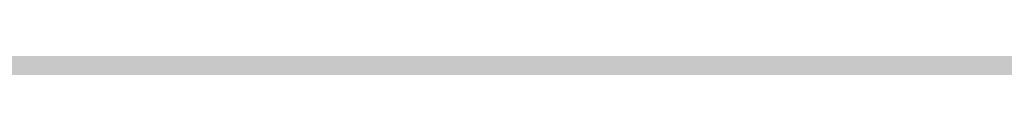
# Model space of a CAD drawing. Units: millimetres. Extents: x 0 to 2267, y 0 to 1823.
# Tile 152 of 256: x 1833.606 to 1838.83, y 1127.355 to 1127.393. Entities that reach past the tile are written whole.
import ezdxf

# ---------------------------------------------------------------- set-up
doc = ezdxf.new("R2010")
doc.units = ezdxf.units.MM
doc.header["$MEASUREMENT"] = 0
doc.layers.add('M-DIMS', color=2, linetype='Continuous', lineweight=25)
doc.layers.add('M-HATC', color=252, linetype='Continuous', lineweight=18)
doc.styles.get("Standard").update_dxf_attribs({"font": 'arial.ttf'})
doc.dimstyles.get("Standard").update_dxf_attribs({"dimtxt": 7, "dimasz": 4, "dimexe": 0.18, "dimexo": 0.0625, "dimgap": 0.09, "dimtad": 0, "dimdec": 0, "dimzin": 0, "dimdsep": 46, "dimtxsty": 'Standard', "dimcen": 0.09, "dimadec": 0, "dimazin": 0, "dimtfac": 1, "dimtdec": 0, "dimtofl": 0, "dimtmove": 0, "dimatfit": 3, "dimfxl": 1, "dimtolj": 1, "dimtzin": 0, "dimarcsym": 0})

# ---------------------------------------------------------------- blocks, each defined once
blk = doc.blocks.new('*D1')
at = {"layer": 'Defpoints', "color": 0, "transparency": 16777216}
for p in [(1593.4289, 1127.4171), (1843.4289, 1127.4171), (1843.4289, 955.6278)]:
    blk.add_point(p, dxfattribs=at)
at = {"layer": 'M-DIMS', "color": 0, "lineweight": -2, "transparency": 16777216}
for p, q in [((1593.4289, 1127.3546), (1593.4289, 955.4478)), ((1843.4289, 1127.3546), (1843.4289, 955.4478)), ((1597.4289, 955.6278), (1710.5582, 955.6278)), ((1839.4289, 955.6278), (1726.2996, 955.6278))]:
    blk.add_line(p, q, dxfattribs=at)
at = {"layer": 'M-DIMS', "color": 0, "transparency": 16777216}
for points in [[(1597.4289, 956.2944), (1597.4289, 954.9611), (1593.4289, 955.6278)], [(1839.4289, 956.2944), (1839.4289, 954.9611), (1843.4289, 955.6278)]]:
    blk.add_solid(points, dxfattribs=at)
at = {"layer": 'M-DIMS', "color": 0, "transparency": 16777216, "insert": (1718.4289, 955.6278), "char_height": 7, "attachment_point": 5}
blk.add_mtext('\\A1;250', dxfattribs=at)

msp = doc.modelspace()

# ---------------------------------------------------------------- hatches: boundary and pattern name
at = {"layer": 'M-HATC'}
h = msp.add_hatch(color=256, dxfattribs=at)
h.dxf.hatch_style = 1
h.paths.add_polyline_path([(2055.771, 1603.062), (1381.0868, 1603.062), (1381.0868, 1598.062), (2055.771, 1598.062)])
h.paths.add_polyline_path([(2055.771, 1598.062), (1381.0868, 1598.062), (1381.0868, 1593.062), (2055.771, 1593.062)])
h.paths.add_polyline_path([(2051.3074, 1536.7609), (1385.5504, 1536.7609), (1385.5504, 1526.7609), (1387.5504, 1526.7609), (1388.5366, 1525.0528), (1385.3319, 1521.2335), (1385.3319, 1521.2226), (2050.2542, 1522.7491), (2048.3212, 1525.0528), (2049.3074, 1526.7609), (2051.3074, 1526.7609)])
edge = h.paths.add_edge_path()
edge.add_arc((1847.5345, 1379.1492), 135, 222.603061, 222.890851, ccw=False)
edge.add_line((1748.1663, 1287.7656), (1683.0921, 1287.7656))
edge.add_arc((1583.7239, 1379.1492), 135, 317.109149, 317.396939, ccw=False)
edge.add_arc((1678.9686, 1290.6707), 5, 222.8909, 317.1091, ccw=False)
edge.add_arc((1774.2133, 1379.1492), 135, 222.603061, 222.890851, ccw=False)
edge.add_line((1674.8451, 1287.7656), (1609.7709, 1287.7656))
edge.add_arc((1510.4027, 1379.1492), 135, 317.109149, 317.396939, ccw=False)
edge.add_arc((1605.6474, 1290.6707), 5, 222.8909, 317.1091, ccw=False)
edge.add_arc((1700.8921, 1379.1492), 135, 222.603061, 222.890851, ccw=False)
edge.add_line((1601.5239, 1287.7656), (1536.4497, 1287.7656))
edge.add_arc((1437.0815, 1379.1492), 135, 317.109149, 317.396939, ccw=False)
edge.add_arc((1532.3262, 1290.6707), 5, 222.8909, 317.1091, ccw=False)
edge.add_arc((1627.5709, 1379.1492), 135, 222.603061, 222.890851, ccw=False)
edge.add_line((1528.2027, 1287.7656), (1505.9289, 1287.7656))
edge.add_spline(control_points=[(1505.9289, 1287.7656), (1504.2622, 1287.7656), (1504.2622, 1282.7656), (1505.9289, 1282.7656)], knot_values=[0, 0, 0, 0, 5, 5, 5, 5], degree=3, periodic=0)
edge.add_line((1505.9289, 1282.7656), (1930.9289, 1282.7656))
edge.add_spline(control_points=[(1930.9289, 1282.7656), (1932.5956, 1282.7656), (1932.5956, 1287.7656), (1930.9289, 1287.7656)], knot_values=[0, 0, 0, 0, 5, 5, 5, 5], degree=3, periodic=0)
edge.add_line((1930.9289, 1287.7656), (1903.0557, 1287.7656))
edge.add_arc((1803.6875, 1379.1492), 135, 317.109149, 317.396939, ccw=False)
edge.add_arc((1898.9322, 1290.6707), 5, 222.8909, 317.1091, ccw=False)
edge.add_arc((1994.1769, 1379.1492), 135, 222.603061, 222.890851, ccw=False)
edge.add_line((1894.8087, 1287.7656), (1829.7345, 1287.7656))
edge.add_arc((1730.3663, 1379.1492), 135, 317.109149, 317.396939, ccw=False)
edge.add_arc((1825.611, 1290.6707), 5, 222.8909, 317.1091, ccw=False)
edge.add_arc((1920.8557, 1379.1492), 135, 222.603061, 222.890851, ccw=False)
edge.add_line((1821.4875, 1287.7656), (1756.4133, 1287.7656))
edge.add_arc((1657.0451, 1379.1492), 135, 317.109149, 317.396939, ccw=False)
edge.add_arc((1752.2898, 1290.6707), 5, 222.8909, 317.1091, ccw=False)
edge = h.paths.add_edge_path()
edge.add_spline(control_points=[(1843.4289, 1227.2475), (1845.0956, 1227.2475), (1845.0956, 1232.2475), (1843.4289, 1232.2475)], knot_values=[0, 0, 0, 0, 5, 5, 5, 5], degree=3, periodic=0)
edge.add_line((1843.4289, 1232.2475), (1593.4289, 1232.2475))
edge.add_spline(control_points=[(1593.4289, 1232.2475), (1591.7622, 1232.2475), (1591.7622, 1227.2475), (1593.4289, 1227.2475)], knot_values=[0, 0, 0, 0, 5, 5, 5, 5], degree=3, periodic=0)
edge.add_line((1593.4289, 1227.2475), (1843.4289, 1227.2475))
h.paths.add_polyline_path([(1905.9289, 1127.4171), (1530.9289, 1127.4171, 0.414214), (1520.9289, 1117.4171), (1530.9289, 1117.4171), (1915.9289, 1117.4171, 0.414214)])
edge = h.paths.add_edge_path()
edge.add_arc((1397.0858, 1498.4078), 12.7299, 90.78215, 190.87871, ccw=False)
edge.add_line((1396.912, 1511.1365), (1428.0097, 1511.3488))
edge.add_line((1428.0097, 1511.3488), (1433.0097, 1511.3488))
edge.add_line((1433.0097, 1511.3488), (1434.439, 1511.3488))
edge.add_arc((1419.474, 1498.0804), 20, 41.561, 74.08211)
edge.add_line((1424.9592, 1517.3135), (1399.9351, 1517.2561))
edge.add_spline(control_points=[(1399.9307, 1517.2561), (1399.884, 1517.2131), (1399.8328, 1517.1689), (1399.7774, 1517.1236)], knot_values=[11.567499, 11.567499, 11.567499, 11.567499, 11.814249, 11.814249, 11.814249, 11.814249], degree=3, periodic=0)
edge.add_spline(control_points=[(1399.6328, 1517.0099), (1399.5831, 1516.9721), (1399.5307, 1516.9338), (1399.4759, 1516.8947)], knot_values=[11.167718, 11.167718, 11.167718, 11.167718, 11.365188, 11.365188, 11.365188, 11.365188], degree=3, periodic=0)
edge.add_spline(control_points=[(1399.3398, 1516.8001), (1399.1514, 1516.6719), (1398.9384, 1516.5377), (1398.704, 1516.3994)], knot_values=[10.376405, 10.376405, 10.376405, 10.376405, 11.00994, 11.00994, 11.00994, 11.00994], degree=3, periodic=0)
edge.add_spline(control_points=[(1398.6572, 1516.3719), (1398.5789, 1516.326), (1398.4983, 1516.2797), (1398.4155, 1516.2331)], knot_values=[10.125175, 10.125175, 10.125175, 10.125175, 10.334406, 10.334406, 10.334406, 10.334406], degree=3, periodic=0)
edge.add_spline(control_points=[(1398.2642, 1516.1487), (1398.196, 1516.1111), (1398.1263, 1516.0732), (1398.0555, 1516.0351)], knot_values=[9.832246, 9.832246, 9.832246, 9.832246, 9.999658, 9.999658, 9.999658, 9.999658], degree=3, periodic=0)
edge.add_spline(control_points=[(1397.9987, 1516.0048), (1397.7312, 1515.8621), (1397.446, 1515.7171), (1397.1466, 1515.5714)], knot_values=[9.161808, 9.161808, 9.161808, 9.161808, 9.787769, 9.787769, 9.787769, 9.787769], degree=3, periodic=0)
edge.add_spline(control_points=[(1397.1466, 1515.5714), (1396.8418, 1515.423), (1396.5222, 1515.274), (1396.1914, 1515.1262)], knot_values=[8.524455, 8.524455, 8.524455, 8.524455, 9.161808, 9.161808, 9.161808, 9.161808], degree=3, periodic=0)
edge.add_spline(control_points=[(1396.0777, 1515.0756), (1395.9854, 1515.0348), (1395.8922, 1514.994), (1395.7983, 1514.9534)], knot_values=[8.275193, 8.275193, 8.275193, 8.275193, 8.451726, 8.451726, 8.451726, 8.451726], degree=3, periodic=0)
edge.add_spline(control_points=[(1395.6018, 1514.8691), (1395.4997, 1514.8257), (1395.3968, 1514.7824), (1395.2932, 1514.7394)], knot_values=[7.962917, 7.962917, 7.962917, 7.962917, 8.152764, 8.152764, 8.152764, 8.152764], degree=3, periodic=0)
edge.add_spline(control_points=[(1395.2116, 1514.7057), (1394.8278, 1514.5475), (1394.4345, 1514.3929), (1394.0364, 1514.2442)], knot_values=[7.21254, 7.21254, 7.21254, 7.21254, 7.913148, 7.913148, 7.913148, 7.913148], degree=3, periodic=0)
edge.add_spline(control_points=[(1394.0364, 1514.2442), (1393.7076, 1514.1214), (1393.3754, 1514.0027), (1393.0427, 1513.8895)], knot_values=[6.633733, 6.633733, 6.633733, 6.633733, 7.21254, 7.21254, 7.21254, 7.21254], degree=3, periodic=0)
edge.add_spline(control_points=[(1392.8214, 1513.815), (1392.7198, 1513.7812), (1392.6181, 1513.7479), (1392.5166, 1513.7152)], knot_values=[6.328796, 6.328796, 6.328796, 6.328796, 6.505493, 6.505493, 6.505493, 6.505493], degree=3, periodic=0)
edge.add_spline(control_points=[(1392.5166, 1513.7152), (1392.3187, 1513.6515), (1392.1212, 1513.59), (1391.9244, 1513.531)], knot_values=[5.984605, 5.984605, 5.984605, 5.984605, 6.328796, 6.328796, 6.328796, 6.328796], degree=3, periodic=0)
edge.add_spline(control_points=[(1391.7915, 1513.4915), (1391.3122, 1513.3501), (1390.8384, 1513.2239), (1390.3784, 1513.1171)], knot_values=[5.066697, 5.066697, 5.066697, 5.066697, 5.907055, 5.907055, 5.907055, 5.907055], degree=3, periodic=0)
edge.add_spline(control_points=[(1390.3784, 1513.1171), (1390.1797, 1513.071), (1389.9836, 1513.0284), (1389.7907, 1512.9899)], knot_values=[4.70367, 4.70367, 4.70367, 4.70367, 5.066695, 5.066695, 5.066695, 5.066695], degree=3, periodic=0)
edge.add_spline(control_points=[(1389.422, 1512.9204), (1389.2459, 1512.8892), (1389.0729, 1512.8617), (1388.9036, 1512.8381)], knot_values=[4.130571, 4.130571, 4.130571, 4.130571, 4.469816, 4.469816, 4.469816, 4.469816], degree=3, periodic=0)
edge.add_spline(control_points=[(1388.9036, 1512.8381), (1388.591, 1512.7946), (1388.2911, 1512.7644), (1388.0071, 1512.7494)], knot_values=[3.504031, 3.504031, 3.504031, 3.504031, 4.130571, 4.130571, 4.130571, 4.130571], degree=3, periodic=0)
edge.add_spline(control_points=[(1387.9356, 1512.7459), (1387.8538, 1512.7423), (1387.7733, 1512.74), (1387.6944, 1512.739)], knot_values=[3.268866, 3.268866, 3.268866, 3.268866, 3.451164, 3.451164, 3.451164, 3.451164], degree=3, periodic=0)
edge.add_spline(control_points=[(1387.3351, 1512.7443), (1387.2076, 1512.7499), (1387.0847, 1512.7597), (1386.967, 1512.7739)], knot_values=[2.670686, 2.670686, 2.670686, 2.670686, 2.984, 2.984, 2.984, 2.984], degree=3, periodic=0)
edge.add_spline(control_points=[(1386.8327, 1512.7922), (1386.8209, 1512.7941), (1386.8092, 1512.7959), (1386.7975, 1512.7979)], knot_values=[2.516981, 2.516981, 2.516981, 2.516981, 2.549528, 2.549528, 2.549528, 2.549528], degree=3, periodic=0)
edge.add_spline(control_points=[(1386.4526, 1512.8735), (1386.4257, 1512.881), (1386.3993, 1512.889), (1386.3733, 1512.8972)], knot_values=[2.095869, 2.095869, 2.095869, 2.095869, 2.17941, 2.17941, 2.17941, 2.17941], degree=3, periodic=0)
edge.add_spline(control_points=[(1386.0691, 1513.0189), (1386.0634, 1513.0217), (1386.0577, 1513.0246), (1386.052, 1513.0275)], knot_values=[1.72453, 1.72453, 1.72453, 1.72453, 1.745933, 1.745933, 1.745933, 1.745933], degree=3, periodic=0)
edge.add_arc((1399.474, 1498.0804), 20, 131.82432, 180)
edge.add_arc((1630.3336, 1505.5484), 250.9708, 181.705176, 236.427975)
edge.add_arc((1605.3399, 1483.3044), 218.7822, 238.660829, 243.34961)
edge.add_arc((1647.0911, 1510.3592), 262.8986, 183.129836, 237.853442, ccw=False)
h.paths.add_polyline_path([(1406.5369, 1391.9644, 0.149382), (1491.5506, 1296.4418, -0.129517)], flags=17)
edge = h.paths.add_edge_path()
edge.add_arc((2037.3838, 1498.0804), 20, 0, 48.26587)
edge.add_spline(control_points=[(2050.6973, 1513.0052), (2050.6512, 1512.9847), (2050.6034, 1512.9655), (2050.5539, 1512.9477)], knot_values=[1.835652, 1.835652, 1.835652, 1.835652, 2.000781, 2.000781, 2.000781, 2.000781], degree=3, periodic=0)
edge.add_spline(control_points=[(2050.4616, 1512.9166), (2050.479, 1512.9221), (2050.4963, 1512.9277), (2050.5133, 1512.9335)], knot_values=[2.045477, 2.045477, 2.045477, 2.045477, 2.101389, 2.101389, 2.101389, 2.101389], degree=3, periodic=0)
edge.add_spline(control_points=[(2050.129, 1512.8342), (2050.1984, 1512.8473), (2050.2657, 1512.8623), (2050.3308, 1512.8792)], knot_values=[2.237629, 2.237629, 2.237629, 2.237629, 2.435841, 2.435841, 2.435841, 2.435841], degree=3, periodic=0)
edge.add_spline(control_points=[(2050.0946, 1512.8278), (2050.1061, 1512.8299), (2050.1176, 1512.832), (2050.129, 1512.8342)], knot_values=[2.435841, 2.435841, 2.435841, 2.435841, 2.468321, 2.468321, 2.468321, 2.468321], degree=3, periodic=0)
edge.add_spline(control_points=[(2049.7843, 1512.7851), (2049.8552, 1512.7922), (2049.9243, 1512.8008), (2049.9917, 1512.8109)], knot_values=[2.563852, 2.563852, 2.563852, 2.563852, 2.748541, 2.748541, 2.748541, 2.748541], degree=3, periodic=0)
edge.add_spline(control_points=[(2049.4052, 1512.7617), (2049.5364, 1512.7653), (2049.6629, 1512.773), (2049.7843, 1512.7851)], knot_values=[2.748541, 2.748541, 2.748541, 2.748541, 3.064882, 3.064882, 3.064882, 3.064882], degree=3, periodic=0)
edge.add_spline(control_points=[(2049.1698, 1512.7597), (2049.2336, 1512.7591), (2049.2965, 1512.7594), (2049.3584, 1512.7606)], knot_values=[3.102309, 3.102309, 3.102309, 3.102309, 3.2503, 3.2503, 3.2503, 3.2503], degree=3, periodic=0)
edge.add_spline(control_points=[(2048.8573, 1512.7691), (2048.9638, 1512.7638), (2049.068, 1512.7606), (2049.1698, 1512.7597)], knot_values=[3.2503, 3.2503, 3.2503, 3.2503, 3.486069, 3.486069, 3.486069, 3.486069], degree=3, periodic=0)
edge.add_spline(control_points=[(2048.6924, 1512.7789), (2048.3729, 1512.8009), (2048.0345, 1512.8411), (2047.6817, 1512.897)], knot_values=[3.606429, 3.606429, 3.606429, 3.606429, 4.2989, 4.2989, 4.2989, 4.2989], degree=3, periodic=0)
edge.add_spline(control_points=[(2047.6817, 1512.897), (2047.5458, 1512.9185), (2047.4077, 1512.9424), (2047.2678, 1512.9685)], knot_values=[4.2989, 4.2989, 4.2989, 4.2989, 4.565769, 4.565769, 4.565769, 4.565769], degree=3, periodic=0)
edge.add_spline(control_points=[(2047.2678, 1512.9685), (2047.1449, 1512.9914), (2047.0207, 1513.016), (2046.8951, 1513.0422)], knot_values=[4.565769, 4.565769, 4.565769, 4.565769, 4.799971, 4.799971, 4.799971, 4.799971], degree=3, periodic=0)
edge.add_spline(control_points=[(2046.8951, 1513.0422), (2046.5286, 1513.1188), (2046.1513, 1513.209), (2045.7676, 1513.3107)], knot_values=[4.799971, 4.799971, 4.799971, 4.799971, 5.483718, 5.483718, 5.483718, 5.483718], degree=3, periodic=0)
edge.add_spline(control_points=[(2045.7676, 1513.3107), (2045.3724, 1513.4154), (2044.9704, 1513.5322), (2044.5662, 1513.6588)], knot_values=[5.483718, 5.483718, 5.483718, 5.483718, 6.187866, 6.187866, 6.187866, 6.187866], degree=3, periodic=0)
edge.add_spline(control_points=[(2044.5662, 1513.6588), (2044.4149, 1513.7061), (2044.2633, 1513.7549), (2044.1116, 1513.8048)], knot_values=[6.187866, 6.187866, 6.187866, 6.187866, 6.451551, 6.451551, 6.451551, 6.451551], degree=3, periodic=0)
edge.add_spline(control_points=[(2044.1116, 1513.8048), (2043.9967, 1513.8427), (2043.8817, 1513.8813), (2043.7668, 1513.9205)], knot_values=[6.451551, 6.451551, 6.451551, 6.451551, 6.651434, 6.651434, 6.651434, 6.651434], degree=3, periodic=0)
edge.add_spline(control_points=[(2043.7668, 1513.9205), (2043.3716, 1514.0554), (2042.9774, 1514.1979), (2042.5886, 1514.3458)], knot_values=[6.651434, 6.651434, 6.651434, 6.651434, 7.338879, 7.338879, 7.338879, 7.338879], degree=3, periodic=0)
edge.add_spline(control_points=[(2042.5886, 1514.3458), (2042.1643, 1514.5071), (2041.7465, 1514.6749), (2041.3409, 1514.846)], knot_values=[7.338879, 7.338879, 7.338879, 7.338879, 8.089209, 8.089209, 8.089209, 8.089209], degree=3, periodic=0)
edge.add_spline(control_points=[(2041.3409, 1514.846), (2041.1028, 1514.9465), (2040.869, 1515.0481), (2040.6405, 1515.1502)], knot_values=[8.089209, 8.089209, 8.089209, 8.089209, 8.529587, 8.529587, 8.529587, 8.529587], degree=3, periodic=0)
edge.add_spline(control_points=[(2040.51, 1515.2089), (2040.0824, 1515.4022), (2039.6747, 1515.5971), (2039.295, 1515.7894)], knot_values=[8.613818, 8.613818, 8.613818, 8.613818, 9.44571, 9.44571, 9.44571, 9.44571], degree=3, periodic=0)
edge.add_spline(control_points=[(2039.295, 1515.7894), (2039.0618, 1515.9075), (2038.8391, 1516.0246), (2038.6288, 1516.1398)], knot_values=[9.44571, 9.44571, 9.44571, 9.44571, 9.956404, 9.956404, 9.956404, 9.956404], degree=3, periodic=0)
edge.add_spline(control_points=[(2038.6288, 1516.1398), (2038.5187, 1516.2001), (2038.4121, 1516.2598), (2038.309, 1516.3189)], knot_values=[9.956404, 9.956404, 9.956404, 9.956404, 10.223542, 10.223542, 10.223542, 10.223542], degree=3, periodic=0)
edge.add_spline(control_points=[(2038.309, 1516.3189), (2038.2138, 1516.3735), (2038.1216, 1516.4276), (2038.0328, 1516.481)], knot_values=[10.223542, 10.223542, 10.223542, 10.223542, 10.47051, 10.47051, 10.47051, 10.47051], degree=3, periodic=0)
edge.add_spline(control_points=[(2038.0328, 1516.481), (2037.7855, 1516.6296), (2037.5639, 1516.773), (2037.3722, 1516.909)], knot_values=[10.47051, 10.47051, 10.47051, 10.47051, 11.15767, 11.15767, 11.15767, 11.15767], degree=3, periodic=0)
edge.add_spline(control_points=[(2037.3722, 1516.909), (2037.2789, 1516.9752), (2037.1927, 1517.0396), (2037.1142, 1517.102)], knot_values=[11.15767, 11.15767, 11.15767, 11.15767, 11.49227, 11.49227, 11.49227, 11.49227], degree=3, periodic=0)
edge.add_spline(control_points=[(2036.8564, 1517.3259), (2036.9148, 1517.2692), (2036.9814, 1517.2103), (2037.0557, 1517.1492)], knot_values=[11.577341, 11.577341, 11.577341, 11.577341, 11.91035, 11.91035, 11.91035, 11.91035], degree=3, periodic=0)
edge.add_spline(control_points=[(2036.8074, 1517.3748), (2036.823, 1517.3587), (2036.8393, 1517.3424), (2036.8564, 1517.3259)], knot_values=[11.91035, 11.91035, 11.91035, 11.91035, 12.007402, 12.007402, 12.007402, 12.007402], degree=3, periodic=0)
edge.add_spline(control_points=[(2036.7017, 1517.494), (2036.7104, 1517.483), (2036.7196, 1517.4719), (2036.7291, 1517.4606)], knot_values=[12.184155, 12.184155, 12.184155, 12.184155, 12.255409, 12.255409, 12.255409, 12.255409], degree=3, periodic=0)
edge.add_spline(control_points=[(2036.6159, 1517.6205), (2036.62, 1517.613), (2036.6243, 1517.6055), (2036.6289, 1517.5979)], knot_values=[12.487913, 12.487913, 12.487913, 12.487913, 12.541035, 12.541035, 12.541035, 12.541035], degree=3, periodic=0)
edge.add_spline(control_points=[(2036.5635, 1517.786), (2036.5637, 1517.7794), (2036.5642, 1517.7726), (2036.565, 1517.7658)], knot_values=[12.911761, 12.911761, 12.911761, 12.911761, 12.968286, 12.968286, 12.968286, 12.968286], degree=3, periodic=0)
edge.add_spline(control_points=[(2036.6166, 1517.9304), (2036.6125, 1517.9259), (2036.6086, 1517.9212), (2036.6049, 1517.9165)], knot_values=[13.382527, 13.382527, 13.382527, 13.382527, 13.433791, 13.433791, 13.433791, 13.433791], degree=3, periodic=0)
edge.add_spline(control_points=[(2036.749, 1518.017), (2036.7361, 1518.0116), (2036.7239, 1518.006), (2036.7124, 1518.0002)], knot_values=[13.726299, 13.726299, 13.726299, 13.726299, 13.809928, 13.809928, 13.809928, 13.809928], degree=3, periodic=0)
edge.add_spline(control_points=[(2036.8604, 1518.0528), (2036.8386, 1518.0474), (2036.8181, 1518.0416), (2036.7988, 1518.0353)], knot_values=[13.910887, 13.910887, 13.910887, 13.910887, 14.02153, 14.02153, 14.02153, 14.02153], degree=3, periodic=0)
edge.add_line((2036.9639, 1518.0804), (2032.3838, 1518.0804))
edge.add_line((2032.3838, 1518.0804), (2027.3838, 1518.0804))
edge.add_line((2027.3838, 1518.0804), (2022.3838, 1518.0804))
edge.add_line((2022.3838, 1518.0804), (2017.3838, 1518.0804))
edge.add_arc((2017.3838, 1498.0804), 20, 90, 138.439)
edge.add_line((2002.4188, 1511.3488), (2003.8481, 1511.3488))
edge.add_line((2003.8481, 1511.3488), (2008.8481, 1511.3488))
edge.add_line((2008.8481, 1511.3488), (2039.772, 1511.1377))
edge.add_arc((2039.772, 1498.4078), 12.7299, -10.87871, 90, ccw=False)
edge.add_arc((1789.7668, 1510.3592), 262.8986, 302.146558, 356.870164, ccw=False)
edge.add_arc((1831.5179, 1483.3044), 218.7822, 296.65039, 301.339171)
edge.add_arc((1806.5242, 1505.5484), 250.9708, 303.572025, 358.294824)
h.paths.add_polyline_path([(2030.321, 1391.9644, -0.129517), (1945.3072, 1296.4418, 0.149382)], flags=17)
edge = h.paths.add_edge_path()
edge.add_spline(control_points=[(2037.2464, 1518.0821), (2037.2898, 1518.081), (2037.3355, 1518.0804), (2037.3838, 1518.0804)], knot_values=[0.000012, 0.000012, 0.000012, 0.000012, 0.144754, 0.144754, 0.144754, 0.144754], degree=3, periodic=0)
edge.add_line((2037.3357, 1518.0804), (2037.0096, 1518.0804))
edge.add_spline(control_points=[(2037.0096, 1518.0804), (2036.9822, 1518.0768), (2036.956, 1518.0727), (2036.9312, 1518.0681)], knot_values=[14.13465, 14.13465, 14.13465, 14.13465, 14.247197, 14.247197, 14.247197, 14.247197], degree=3, periodic=0)
edge.add_spline(control_points=[(2036.9312, 1518.0681), (2036.9276, 1518.0674), (2036.9241, 1518.0667), (2036.9205, 1518.0661)], knot_values=[14.118315, 14.118315, 14.118315, 14.118315, 14.13465, 14.13465, 14.13465, 14.13465], degree=3, periodic=0)
edge.add_spline(control_points=[(2036.9205, 1518.0661), (2036.9118, 1518.0644), (2036.9032, 1518.0626), (2036.8948, 1518.0608)], knot_values=[14.078086, 14.078086, 14.078086, 14.078086, 14.118315, 14.118315, 14.118315, 14.118315], degree=3, periodic=0)
edge.add_spline(control_points=[(2036.8948, 1518.0608), (2036.883, 1518.0583), (2036.8716, 1518.0556), (2036.8604, 1518.0528)], knot_values=[14.02153, 14.02153, 14.02153, 14.02153, 14.078086, 14.078086, 14.078086, 14.078086], degree=3, periodic=0)
edge.add_spline(control_points=[(2036.8604, 1518.0528), (2036.8386, 1518.0474), (2036.8181, 1518.0416), (2036.7988, 1518.0353)], knot_values=[13.910887, 13.910887, 13.910887, 13.910887, 14.02153, 14.02153, 14.02153, 14.02153], degree=3, periodic=0)
edge.add_spline(control_points=[(2036.7988, 1518.0353), (2036.7981, 1518.035), (2036.7974, 1518.0348), (2036.7967, 1518.0346)], knot_values=[13.906906, 13.906906, 13.906906, 13.906906, 13.910887, 13.910887, 13.910887, 13.910887], degree=3, periodic=0)
edge.add_spline(control_points=[(2036.7967, 1518.0346), (2036.7882, 1518.0318), (2036.7799, 1518.0289), (2036.7719, 1518.0259)], knot_values=[13.857826, 13.857826, 13.857826, 13.857826, 13.906906, 13.906906, 13.906906, 13.906906], degree=3, periodic=0)
edge.add_spline(control_points=[(2036.7719, 1518.0259), (2036.764, 1518.023), (2036.7564, 1518.02), (2036.749, 1518.017)], knot_values=[13.809928, 13.809928, 13.809928, 13.809928, 13.857826, 13.857826, 13.857826, 13.857826], degree=3, periodic=0)
edge.add_spline(control_points=[(2036.749, 1518.017), (2036.7361, 1518.0116), (2036.7239, 1518.006), (2036.7124, 1518.0002)], knot_values=[13.726299, 13.726299, 13.726299, 13.726299, 13.809928, 13.809928, 13.809928, 13.809928], degree=3, periodic=0)
edge.add_spline(control_points=[(2036.7124, 1518.0002), (2036.7121, 1518), (2036.7118, 1517.9999), (2036.7115, 1517.9997)], knot_values=[13.723993, 13.723993, 13.723993, 13.723993, 13.726299, 13.726299, 13.726299, 13.726299], degree=3, periodic=0)
edge.add_spline(control_points=[(2036.7115, 1517.9997), (2036.7063, 1517.9971), (2036.7013, 1517.9944), (2036.6965, 1517.9917)], knot_values=[13.686536, 13.686536, 13.686536, 13.686536, 13.723993, 13.723993, 13.723993, 13.723993], degree=3, periodic=0)
edge.add_spline(control_points=[(2036.6965, 1517.9917), (2036.6919, 1517.9891), (2036.6874, 1517.9865), (2036.6831, 1517.9839)], knot_values=[13.651251, 13.651251, 13.651251, 13.651251, 13.686536, 13.686536, 13.686536, 13.686536], degree=3, periodic=0)
edge.add_spline(control_points=[(2036.6831, 1517.9839), (2036.6764, 1517.9798), (2036.67, 1517.9757), (2036.6639, 1517.9714)], knot_values=[13.596804, 13.596804, 13.596804, 13.596804, 13.651251, 13.651251, 13.651251, 13.651251], degree=3, periodic=0)
edge.add_spline(control_points=[(2036.6639, 1517.9714), (2036.6636, 1517.9712), (2036.6633, 1517.9709), (2036.6629, 1517.9707)], knot_values=[13.593956, 13.593956, 13.593956, 13.593956, 13.596804, 13.596804, 13.596804, 13.596804], degree=3, periodic=0)
edge.add_spline(control_points=[(2036.6629, 1517.9707), (2036.6603, 1517.9689), (2036.6577, 1517.967), (2036.6552, 1517.9651)], knot_values=[13.570322, 13.570322, 13.570322, 13.570322, 13.593956, 13.593956, 13.593956, 13.593956], degree=3, periodic=0)
edge.add_spline(control_points=[(2036.6552, 1517.9651), (2036.6525, 1517.9631), (2036.6499, 1517.9611), (2036.6474, 1517.9591)], knot_values=[13.545477, 13.545477, 13.545477, 13.545477, 13.570322, 13.570322, 13.570322, 13.570322], degree=3, periodic=0)
edge.add_spline(control_points=[(2036.6474, 1517.9591), (2036.6472, 1517.9589), (2036.6471, 1517.9588), (2036.6469, 1517.9587)], knot_values=[13.543931, 13.543931, 13.543931, 13.543931, 13.545477, 13.545477, 13.545477, 13.545477], degree=3, periodic=0)
edge.add_spline(control_points=[(2036.6469, 1517.9587), (2036.6412, 1517.9541), (2036.6358, 1517.9494), (2036.6307, 1517.9447)], knot_values=[13.488237, 13.488237, 13.488237, 13.488237, 13.543931, 13.543931, 13.543931, 13.543931], degree=3, periodic=0)
edge.add_spline(control_points=[(2036.6307, 1517.9447), (2036.6282, 1517.9423), (2036.6257, 1517.9399), (2036.6233, 1517.9374)], knot_values=[13.460307, 13.460307, 13.460307, 13.460307, 13.488237, 13.488237, 13.488237, 13.488237], degree=3, periodic=0)
edge.add_spline(control_points=[(2036.6233, 1517.9374), (2036.6215, 1517.9356), (2036.6198, 1517.9338), (2036.6181, 1517.932)], knot_values=[13.439712, 13.439712, 13.439712, 13.439712, 13.460307, 13.460307, 13.460307, 13.460307], degree=3, periodic=0)
edge.add_spline(control_points=[(2036.6181, 1517.932), (2036.6176, 1517.9315), (2036.6171, 1517.9309), (2036.6166, 1517.9304)], knot_values=[13.433791, 13.433791, 13.433791, 13.433791, 13.439712, 13.439712, 13.439712, 13.439712], degree=3, periodic=0)
edge.add_spline(control_points=[(2036.6166, 1517.9304), (2036.6125, 1517.9259), (2036.6086, 1517.9212), (2036.6049, 1517.9165)], knot_values=[13.382527, 13.382527, 13.382527, 13.382527, 13.433791, 13.433791, 13.433791, 13.433791], degree=3, periodic=0)
edge.add_spline(control_points=[(2036.6049, 1517.9165), (2036.6026, 1517.9135), (2036.6004, 1517.9104), (2036.5982, 1517.9074)], knot_values=[13.350017, 13.350017, 13.350017, 13.350017, 13.382527, 13.382527, 13.382527, 13.382527], degree=3, periodic=0)
edge.add_spline(control_points=[(2036.5982, 1517.9074), (2036.5972, 1517.9059), (2036.5962, 1517.9043), (2036.5952, 1517.9028)], knot_values=[13.333922, 13.333922, 13.333922, 13.333922, 13.350017, 13.350017, 13.350017, 13.350017], degree=3, periodic=0)
edge.add_spline(control_points=[(2036.5952, 1517.9028), (2036.5945, 1517.9018), (2036.5939, 1517.9009), (2036.5933, 1517.8999)], knot_values=[13.323828, 13.323828, 13.323828, 13.323828, 13.333922, 13.333922, 13.333922, 13.333922], degree=3, periodic=0)
edge.add_spline(control_points=[(2036.5933, 1517.8999), (2036.5905, 1517.8955), (2036.5879, 1517.8909), (2036.5855, 1517.8864)], knot_values=[13.277545, 13.277545, 13.277545, 13.277545, 13.323828, 13.323828, 13.323828, 13.323828], degree=3, periodic=0)
edge.add_spline(control_points=[(2036.5855, 1517.8864), (2036.5836, 1517.8827), (2036.5817, 1517.8789), (2036.5801, 1517.8751)], knot_values=[13.240119, 13.240119, 13.240119, 13.240119, 13.277545, 13.277545, 13.277545, 13.277545], degree=3, periodic=0)
edge.add_spline(control_points=[(2036.5801, 1517.8751), (2036.5795, 1517.8739), (2036.579, 1517.8727), (2036.5785, 1517.8715)], knot_values=[13.228211, 13.228211, 13.228211, 13.228211, 13.240119, 13.240119, 13.240119, 13.240119], degree=3, periodic=0)
edge.add_spline(control_points=[(2036.5785, 1517.8715), (2036.578, 1517.8702), (2036.5774, 1517.869), (2036.5769, 1517.8677)], knot_values=[13.215717, 13.215717, 13.215717, 13.215717, 13.228211, 13.228211, 13.228211, 13.228211], degree=3, periodic=0)
edge.add_spline(control_points=[(2036.5769, 1517.8677), (2036.5755, 1517.864), (2036.5741, 1517.8603), (2036.5729, 1517.8565)], knot_values=[13.179847, 13.179847, 13.179847, 13.179847, 13.215717, 13.215717, 13.215717, 13.215717], degree=3, periodic=0)
edge.add_spline(control_points=[(2036.5729, 1517.8565), (2036.5713, 1517.8515), (2036.5699, 1517.8464), (2036.5687, 1517.8413)], knot_values=[13.132017, 13.132017, 13.132017, 13.132017, 13.179847, 13.179847, 13.179847, 13.179847], degree=3, periodic=0)
edge.add_spline(control_points=[(2036.5687, 1517.8413), (2036.5684, 1517.8402), (2036.5682, 1517.8392), (2036.568, 1517.8382)], knot_values=[13.122482, 13.122482, 13.122482, 13.122482, 13.132017, 13.132017, 13.132017, 13.132017], degree=3, periodic=0)
edge.add_spline(control_points=[(2036.568, 1517.8382), (2036.5676, 1517.8363), (2036.5672, 1517.8345), (2036.5669, 1517.8327)], knot_values=[13.105592, 13.105592, 13.105592, 13.105592, 13.122482, 13.122482, 13.122482, 13.122482], degree=3, periodic=0)
edge.add_spline(control_points=[(2036.5669, 1517.8327), (2036.5662, 1517.8292), (2036.5657, 1517.8257), (2036.5652, 1517.8222)], knot_values=[13.074063, 13.074063, 13.074063, 13.074063, 13.105592, 13.105592, 13.105592, 13.105592], degree=3, periodic=0)
edge.add_spline(control_points=[(2036.5652, 1517.8222), (2036.5652, 1517.8222), (2036.5652, 1517.8222), (2036.5652, 1517.8222)], knot_values=[13.074043, 13.074043, 13.074043, 13.074043, 13.074063, 13.074063, 13.074063, 13.074063], degree=3, periodic=0)
edge.add_spline(control_points=[(2036.5652, 1517.8222), (2036.5644, 1517.8164), (2036.5639, 1517.8106), (2036.5636, 1517.8046)], knot_values=[13.021884, 13.021884, 13.021884, 13.021884, 13.074043, 13.074043, 13.074043, 13.074043], degree=3, periodic=0)
edge.add_spline(control_points=[(2036.5636, 1517.8046), (2036.5636, 1517.804), (2036.5636, 1517.8034), (2036.5635, 1517.8028)], knot_values=[13.01674, 13.01674, 13.01674, 13.01674, 13.021884, 13.021884, 13.021884, 13.021884], degree=3, periodic=0)
edge.add_spline(control_points=[(2036.5635, 1517.8028), (2036.5634, 1517.8005), (2036.5634, 1517.7982), (2036.5634, 1517.7958)], knot_values=[12.996438, 12.996438, 12.996438, 12.996438, 13.01674, 13.01674, 13.01674, 13.01674], degree=3, periodic=0)
edge.add_spline(control_points=[(2036.5634, 1517.7958), (2036.5633, 1517.7926), (2036.5634, 1517.7893), (2036.5635, 1517.786)], knot_values=[12.968286, 12.968286, 12.968286, 12.968286, 12.996438, 12.996438, 12.996438, 12.996438], degree=3, periodic=0)
edge.add_spline(control_points=[(2036.5635, 1517.786), (2036.5637, 1517.7794), (2036.5642, 1517.7726), (2036.565, 1517.7658)], knot_values=[12.911761, 12.911761, 12.911761, 12.911761, 12.968286, 12.968286, 12.968286, 12.968286], degree=3, periodic=0)
edge.add_spline(control_points=[(2036.565, 1517.7658), (2036.565, 1517.7657), (2036.565, 1517.7656), (2036.565, 1517.7656)], knot_values=[12.911017, 12.911017, 12.911017, 12.911017, 12.911761, 12.911761, 12.911761, 12.911761], degree=3, periodic=0)
edge.add_spline(control_points=[(2036.565, 1517.7656), (2036.5654, 1517.7625), (2036.5658, 1517.7593), (2036.5663, 1517.7562)], knot_values=[12.88528, 12.88528, 12.88528, 12.88528, 12.911017, 12.911017, 12.911017, 12.911017], degree=3, periodic=0)
edge.add_spline(control_points=[(2036.5663, 1517.7562), (2036.5667, 1517.7534), (2036.5672, 1517.7506), (2036.5677, 1517.7478)], knot_values=[12.862519, 12.862519, 12.862519, 12.862519, 12.88528, 12.88528, 12.88528, 12.88528], degree=3, periodic=0)
edge.add_spline(control_points=[(2036.5677, 1517.7478), (2036.5678, 1517.7474), (2036.5679, 1517.7469), (2036.568, 1517.7465)], knot_values=[12.858885, 12.858885, 12.858885, 12.858885, 12.862519, 12.862519, 12.862519, 12.862519], degree=3, periodic=0)
edge.add_spline(control_points=[(2036.568, 1517.7465), (2036.5692, 1517.7399), (2036.5707, 1517.7332), (2036.5724, 1517.7264)], knot_values=[12.8053, 12.8053, 12.8053, 12.8053, 12.858885, 12.858885, 12.858885, 12.858885], degree=3, periodic=0)
edge.add_spline(control_points=[(2036.5724, 1517.7264), (2036.5734, 1517.7226), (2036.5745, 1517.7187), (2036.5756, 1517.7149)], knot_values=[12.775176, 12.775176, 12.775176, 12.775176, 12.8053, 12.8053, 12.8053, 12.8053], degree=3, periodic=0)
edge.add_spline(control_points=[(2036.5756, 1517.7149), (2036.5763, 1517.7125), (2036.577, 1517.7102), (2036.5778, 1517.7078)], knot_values=[12.756759, 12.756759, 12.756759, 12.756759, 12.775176, 12.775176, 12.775176, 12.775176], degree=3, periodic=0)
edge.add_spline(control_points=[(2036.5778, 1517.7078), (2036.5781, 1517.7067), (2036.5784, 1517.7057), (2036.5787, 1517.7047)], knot_values=[12.748742, 12.748742, 12.748742, 12.748742, 12.756759, 12.756759, 12.756759, 12.756759], degree=3, periodic=0)
edge.add_spline(control_points=[(2036.5787, 1517.7047), (2036.5808, 1517.6983), (2036.5831, 1517.6919), (2036.5856, 1517.6854)], knot_values=[12.69959, 12.69959, 12.69959, 12.69959, 12.748742, 12.748742, 12.748742, 12.748742], degree=3, periodic=0)
edge.add_spline(control_points=[(2036.5856, 1517.6854), (2036.5876, 1517.68), (2036.5898, 1517.6746), (2036.5921, 1517.6692)], knot_values=[12.659038, 12.659038, 12.659038, 12.659038, 12.69959, 12.69959, 12.69959, 12.69959], degree=3, periodic=0)
edge.add_spline(control_points=[(2036.5921, 1517.6692), (2036.594, 1517.6648), (2036.5959, 1517.6605), (2036.5979, 1517.6561)], knot_values=[12.626806, 12.626806, 12.626806, 12.626806, 12.659038, 12.659038, 12.659038, 12.659038], degree=3, periodic=0)
edge.add_spline(control_points=[(2036.5979, 1517.6561), (2036.5984, 1517.6551), (2036.5989, 1517.6541), (2036.5993, 1517.6531)], knot_values=[12.619394, 12.619394, 12.619394, 12.619394, 12.626806, 12.626806, 12.626806, 12.626806], degree=3, periodic=0)
edge.add_spline(control_points=[(2036.5993, 1517.6531), (2036.6043, 1517.6424), (2036.6099, 1517.6315), (2036.6159, 1517.6205)], knot_values=[12.541039, 12.541039, 12.541039, 12.541039, 12.619394, 12.619394, 12.619394, 12.619394], degree=3, periodic=0)
edge.add_spline(control_points=[(2036.6159, 1517.6205), (2036.6159, 1517.6205), (2036.6159, 1517.6205), (2036.6159, 1517.6205)], knot_values=[12.541035, 12.541035, 12.541035, 12.541035, 12.541039, 12.541039, 12.541039, 12.541039], degree=3, periodic=0)
edge.add_spline(control_points=[(2036.6159, 1517.6205), (2036.62, 1517.613), (2036.6243, 1517.6055), (2036.6289, 1517.5979)], knot_values=[12.487913, 12.487913, 12.487913, 12.487913, 12.541035, 12.541035, 12.541035, 12.541035], degree=3, periodic=0)
edge.add_spline(control_points=[(2036.6289, 1517.5979), (2036.6326, 1517.5916), (2036.6365, 1517.5853), (2036.6406, 1517.5789)], knot_values=[12.443982, 12.443982, 12.443982, 12.443982, 12.487913, 12.487913, 12.487913, 12.487913], degree=3, periodic=0)
edge.add_spline(control_points=[(2036.6406, 1517.5789), (2036.6414, 1517.5776), (2036.6423, 1517.5763), (2036.6431, 1517.5749)], knot_values=[12.434996, 12.434996, 12.434996, 12.434996, 12.443982, 12.443982, 12.443982, 12.443982], degree=3, periodic=0)
edge.add_spline(control_points=[(2036.6431, 1517.5749), (2036.6531, 1517.5596), (2036.6639, 1517.5439), (2036.6756, 1517.528)], knot_values=[12.329647, 12.329647, 12.329647, 12.329647, 12.434996, 12.434996, 12.434996, 12.434996], degree=3, periodic=0)
edge.add_spline(control_points=[(2036.6756, 1517.528), (2036.6839, 1517.5168), (2036.6925, 1517.5055), (2036.7017, 1517.494)], knot_values=[12.255409, 12.255409, 12.255409, 12.255409, 12.329647, 12.329647, 12.329647, 12.329647], degree=3, periodic=0)
edge.add_spline(control_points=[(2036.7017, 1517.494), (2036.7104, 1517.483), (2036.7196, 1517.4719), (2036.7291, 1517.4606)], knot_values=[12.184155, 12.184155, 12.184155, 12.184155, 12.255409, 12.255409, 12.255409, 12.255409], degree=3, periodic=0)
edge.add_spline(control_points=[(2036.7291, 1517.4606), (2036.7436, 1517.4435), (2036.759, 1517.4262), (2036.7753, 1517.4085)], knot_values=[12.075961, 12.075961, 12.075961, 12.075961, 12.184155, 12.184155, 12.184155, 12.184155], degree=3, periodic=0)
edge.add_spline(control_points=[(2036.7753, 1517.4085), (2036.7763, 1517.4075), (2036.7773, 1517.4064), (2036.7783, 1517.4054)], knot_values=[12.069502, 12.069502, 12.069502, 12.069502, 12.075961, 12.075961, 12.075961, 12.075961], degree=3, periodic=0)
edge.add_spline(control_points=[(2036.7783, 1517.4054), (2036.7877, 1517.3953), (2036.7974, 1517.385), (2036.8074, 1517.3748)], knot_values=[12.007402, 12.007402, 12.007402, 12.007402, 12.069502, 12.069502, 12.069502, 12.069502], degree=3, periodic=0)
edge.add_spline(control_points=[(2036.8074, 1517.3748), (2036.823, 1517.3587), (2036.8393, 1517.3424), (2036.8564, 1517.3259)], knot_values=[11.91035, 11.91035, 11.91035, 11.91035, 12.007402, 12.007402, 12.007402, 12.007402], degree=3, periodic=0)
edge.add_spline(control_points=[(2036.8564, 1517.3259), (2036.9148, 1517.2692), (2036.9814, 1517.2103), (2037.0557, 1517.1492)], knot_values=[11.577341, 11.577341, 11.577341, 11.577341, 11.91035, 11.91035, 11.91035, 11.91035], degree=3, periodic=0)
edge.add_spline(control_points=[(2037.0557, 1517.1492), (2037.0747, 1517.1336), (2037.0942, 1517.1179), (2037.1142, 1517.102)], knot_values=[11.49227, 11.49227, 11.49227, 11.49227, 11.577341, 11.577341, 11.577341, 11.577341], degree=3, periodic=0)
edge.add_spline(control_points=[(2037.1142, 1517.102), (2037.1927, 1517.0396), (2037.2789, 1516.9752), (2037.3722, 1516.909)], knot_values=[11.15767, 11.15767, 11.15767, 11.15767, 11.49227, 11.49227, 11.49227, 11.49227], degree=3, periodic=0)
edge.add_spline(control_points=[(2037.3722, 1516.909), (2037.5639, 1516.773), (2037.7855, 1516.6296), (2038.0328, 1516.481)], knot_values=[10.47051, 10.47051, 10.47051, 10.47051, 11.15767, 11.15767, 11.15767, 11.15767], degree=3, periodic=0)
edge.add_spline(control_points=[(2038.0328, 1516.481), (2038.1216, 1516.4276), (2038.2138, 1516.3735), (2038.309, 1516.3189)], knot_values=[10.223542, 10.223542, 10.223542, 10.223542, 10.47051, 10.47051, 10.47051, 10.47051], degree=3, periodic=0)
edge.add_spline(control_points=[(2038.309, 1516.3189), (2038.4121, 1516.2598), (2038.5187, 1516.2001), (2038.6288, 1516.1398)], knot_values=[9.956404, 9.956404, 9.956404, 9.956404, 10.223542, 10.223542, 10.223542, 10.223542], degree=3, periodic=0)
edge.add_spline(control_points=[(2038.6288, 1516.1398), (2038.8391, 1516.0246), (2039.0618, 1515.9075), (2039.295, 1515.7894)], knot_values=[9.44571, 9.44571, 9.44571, 9.44571, 9.956404, 9.956404, 9.956404, 9.956404], degree=3, periodic=0)
edge.add_spline(control_points=[(2039.295, 1515.7894), (2039.6747, 1515.5971), (2040.0824, 1515.4022), (2040.51, 1515.2089)], knot_values=[8.613818, 8.613818, 8.613818, 8.613818, 9.44571, 9.44571, 9.44571, 9.44571], degree=3, periodic=0)
edge.add_spline(control_points=[(2040.51, 1515.2089), (2040.5533, 1515.1893), (2040.5968, 1515.1697), (2040.6405, 1515.1502)], knot_values=[8.529587, 8.529587, 8.529587, 8.529587, 8.613818, 8.613818, 8.613818, 8.613818], degree=3, periodic=0)
edge.add_spline(control_points=[(2040.6405, 1515.1502), (2040.869, 1515.0481), (2041.1028, 1514.9465), (2041.3409, 1514.846)], knot_values=[8.089209, 8.089209, 8.089209, 8.089209, 8.529587, 8.529587, 8.529587, 8.529587], degree=3, periodic=0)
edge.add_spline(control_points=[(2041.3409, 1514.846), (2041.7465, 1514.6749), (2042.1643, 1514.5071), (2042.5886, 1514.3458)], knot_values=[7.338879, 7.338879, 7.338879, 7.338879, 8.089209, 8.089209, 8.089209, 8.089209], degree=3, periodic=0)
edge.add_spline(control_points=[(2042.5886, 1514.3458), (2042.9774, 1514.1979), (2043.3716, 1514.0554), (2043.7668, 1513.9205)], knot_values=[6.651434, 6.651434, 6.651434, 6.651434, 7.338879, 7.338879, 7.338879, 7.338879], degree=3, periodic=0)
edge.add_spline(control_points=[(2043.7668, 1513.9205), (2043.8817, 1513.8813), (2043.9967, 1513.8427), (2044.1116, 1513.8048)], knot_values=[6.451551, 6.451551, 6.451551, 6.451551, 6.651434, 6.651434, 6.651434, 6.651434], degree=3, periodic=0)
edge.add_spline(control_points=[(2044.1116, 1513.8048), (2044.2633, 1513.7549), (2044.4149, 1513.7061), (2044.5662, 1513.6588)], knot_values=[6.187866, 6.187866, 6.187866, 6.187866, 6.451551, 6.451551, 6.451551, 6.451551], degree=3, periodic=0)
edge.add_spline(control_points=[(2044.5662, 1513.6588), (2044.9704, 1513.5322), (2045.3724, 1513.4154), (2045.7676, 1513.3107)], knot_values=[5.483718, 5.483718, 5.483718, 5.483718, 6.187866, 6.187866, 6.187866, 6.187866], degree=3, periodic=0)
edge.add_spline(control_points=[(2045.7676, 1513.3107), (2046.1513, 1513.209), (2046.5286, 1513.1188), (2046.8951, 1513.0422)], knot_values=[4.799971, 4.799971, 4.799971, 4.799971, 5.483718, 5.483718, 5.483718, 5.483718], degree=3, periodic=0)
edge.add_spline(control_points=[(2046.8951, 1513.0422), (2047.0207, 1513.016), (2047.1449, 1512.9914), (2047.2678, 1512.9685)], knot_values=[4.565769, 4.565769, 4.565769, 4.565769, 4.799971, 4.799971, 4.799971, 4.799971], degree=3, periodic=0)
edge.add_spline(control_points=[(2047.2678, 1512.9685), (2047.4077, 1512.9424), (2047.5458, 1512.9185), (2047.6817, 1512.897)], knot_values=[4.2989, 4.2989, 4.2989, 4.2989, 4.565769, 4.565769, 4.565769, 4.565769], degree=3, periodic=0)
edge.add_spline(control_points=[(2047.6817, 1512.897), (2048.0345, 1512.8411), (2048.3729, 1512.8009), (2048.6924, 1512.7789)], knot_values=[3.606429, 3.606429, 3.606429, 3.606429, 4.2989, 4.2989, 4.2989, 4.2989], degree=3, periodic=0)
edge.add_spline(control_points=[(2048.6924, 1512.7789), (2048.7479, 1512.7751), (2048.8029, 1512.7718), (2048.8573, 1512.7691)], knot_values=[3.486069, 3.486069, 3.486069, 3.486069, 3.606429, 3.606429, 3.606429, 3.606429], degree=3, periodic=0)
edge.add_spline(control_points=[(2048.8573, 1512.7691), (2048.9638, 1512.7638), (2049.068, 1512.7606), (2049.1698, 1512.7597)], knot_values=[3.2503, 3.2503, 3.2503, 3.2503, 3.486069, 3.486069, 3.486069, 3.486069], degree=3, periodic=0)
edge.add_spline(control_points=[(2049.1698, 1512.7597), (2049.2336, 1512.7591), (2049.2965, 1512.7594), (2049.3584, 1512.7606)], knot_values=[3.102309, 3.102309, 3.102309, 3.102309, 3.2503, 3.2503, 3.2503, 3.2503], degree=3, periodic=0)
edge.add_spline(control_points=[(2049.3584, 1512.7606), (2049.3741, 1512.7609), (2049.3897, 1512.7613), (2049.4052, 1512.7617)], knot_values=[3.064882, 3.064882, 3.064882, 3.064882, 3.102309, 3.102309, 3.102309, 3.102309], degree=3, periodic=0)
edge.add_spline(control_points=[(2049.4052, 1512.7617), (2049.5364, 1512.7653), (2049.6629, 1512.773), (2049.7843, 1512.7851)], knot_values=[2.748541, 2.748541, 2.748541, 2.748541, 3.064882, 3.064882, 3.064882, 3.064882], degree=3, periodic=0)
edge.add_spline(control_points=[(2049.7843, 1512.7851), (2049.8552, 1512.7922), (2049.9243, 1512.8008), (2049.9917, 1512.8109)], knot_values=[2.563852, 2.563852, 2.563852, 2.563852, 2.748541, 2.748541, 2.748541, 2.748541], degree=3, periodic=0)
edge.add_spline(control_points=[(2049.9917, 1512.8109), (2050.0265, 1512.8161), (2050.0608, 1512.8218), (2050.0946, 1512.8278)], knot_values=[2.468321, 2.468321, 2.468321, 2.468321, 2.563852, 2.563852, 2.563852, 2.563852], degree=3, periodic=0)
edge.add_spline(control_points=[(2050.0946, 1512.8278), (2050.1061, 1512.8299), (2050.1176, 1512.832), (2050.129, 1512.8342)], knot_values=[2.435841, 2.435841, 2.435841, 2.435841, 2.468321, 2.468321, 2.468321, 2.468321], degree=3, periodic=0)
edge.add_spline(control_points=[(2050.129, 1512.8342), (2050.1984, 1512.8473), (2050.2657, 1512.8623), (2050.3308, 1512.8792)], knot_values=[2.237629, 2.237629, 2.237629, 2.237629, 2.435841, 2.435841, 2.435841, 2.435841], degree=3, periodic=0)
edge.add_spline(control_points=[(2050.3308, 1512.8792), (2050.3754, 1512.8908), (2050.4191, 1512.9032), (2050.4616, 1512.9166)], knot_values=[2.101389, 2.101389, 2.101389, 2.101389, 2.237629, 2.237629, 2.237629, 2.237629], degree=3, periodic=0)
edge.add_spline(control_points=[(2050.4616, 1512.9166), (2050.479, 1512.9221), (2050.4963, 1512.9277), (2050.5133, 1512.9335)], knot_values=[2.045477, 2.045477, 2.045477, 2.045477, 2.101389, 2.101389, 2.101389, 2.101389], degree=3, periodic=0)
edge.add_spline(control_points=[(2050.5133, 1512.9335), (2050.527, 1512.9382), (2050.5405, 1512.9429), (2050.5539, 1512.9477)], knot_values=[2.000781, 2.000781, 2.000781, 2.000781, 2.045477, 2.045477, 2.045477, 2.045477], degree=3, periodic=0)
edge.add_spline(control_points=[(2050.5539, 1512.9477), (2050.6034, 1512.9655), (2050.6512, 1512.9847), (2050.6973, 1513.0052)], knot_values=[1.835652, 1.835652, 1.835652, 1.835652, 2.000781, 2.000781, 2.000781, 2.000781], degree=3, periodic=0)
edge.add_arc((2037.3838, 1498.0804), 20, 48.26587, 90.12993)
edge = h.paths.add_edge_path(flags=16)
edge.add_spline(control_points=[(1386.1389, 1512.9859), (1388.92, 1511.7395), (1398.0387, 1515.5187), (1399.9307, 1517.2561)], knot_values=[1.831046, 1.831046, 1.831046, 1.831046, 11.814249, 11.814249, 11.814249, 11.814249], degree=3, periodic=0)
edge.add_line((1399.9307, 1517.2561), (1393.7435, 1517.2419))
edge.add_arc((1399.474, 1498.0804), 20, 106.6501, 131.8173)

# ---------------------------------------------------------------- dimensions: what is measured, and where the dimension line sits
at = {"layer": 'M-DIMS'}
dim = msp.add_linear_dim(base=(1843.4289, 955.6278), p1=(1593.4289, 1127.4171), p2=(1843.4289, 1127.4171), dimstyle='Standard', override={"dimclrd": 0, "dimclre": 0, "dimclrt": 0}, dxfattribs=at)
dim.commit()
dim.dimension.update_dxf_attribs({"geometry": '*D1', "text_midpoint": (1718.4289, 955.6278)})

doc.saveas('drawing.dxf')
